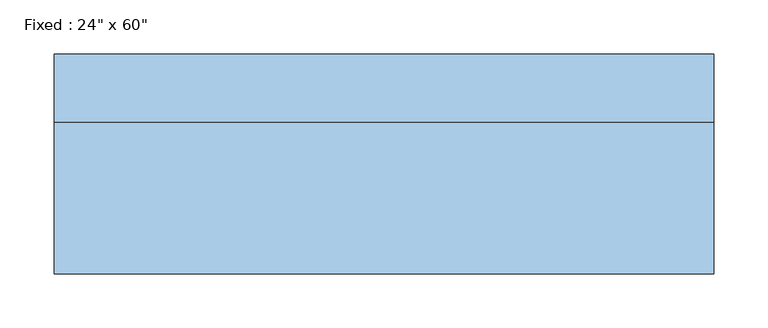
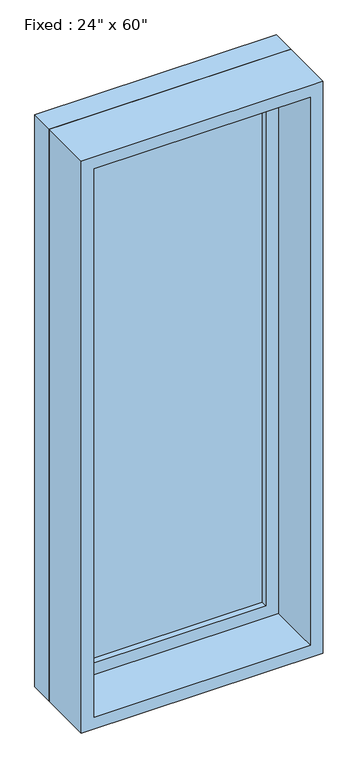
"""IFC4 building model written with IfcOpenShell, lengths in millimetres: window geometry."""

from ifc_helpers import new_model, si_unit, frame, origin, place, context, project, spatial, polyline, outline, extrude, source, transform, mapped, element, save


def window_8561b6b6(model_context):
    return source(origin(), model_context, "Body", "SweptSolid", [
        extrude(outline(polyline([(203.2, 53.975), (-279.4, 53.975), (-279.4, 66.675), (203.2, 66.675), (203.2, 53.975)])), frame((0.0, 0.0, 977.9), z_axis=(0.0, 0.0, 1.0), x_axis=(1.0, 0.0, 0.0)), (0.0, 0.0, 1.0), 1397.0),
        extrude(outline(polyline([(2419.35, -323.85), (933.45, -323.85), (933.45, 247.65), (2419.35, 247.65), (2419.35, -323.85)]), holes=[polyline([(2374.9, -279.4), (2374.9, 203.2), (977.9, 203.2), (977.9, -279.4), (2374.9, -279.4)])]), frame((0.0, 38.1, 0.0), z_axis=(0.0, 1.0, 0.0), x_axis=(0.0, 0.0, 1.0)), (0.0, 0.0, 1.0), 44.45),
        extrude(outline(polyline([(2438.4, -342.9), (914.4, -342.9), (914.4, 266.7), (2438.4, 266.7), (2438.4, -342.9)]), holes=[polyline([(2406.65, -311.15), (2406.65, 234.95), (946.15, 234.95), (946.15, -311.15), (2406.65, -311.15)])]), frame((0.0, -101.6, 0.0), z_axis=(0.0, 1.0, 0.0), x_axis=(0.0, 0.0, 1.0)), (0.0, 0.0, 1.0), 139.7),
        extrude(outline(polyline([(2438.4, 266.7), (2438.4, -342.9), (914.4, -342.9), (914.4, 266.7), (2438.4, 266.7)]), holes=[polyline([(2419.35, 247.65), (933.45, 247.65), (933.45, -323.85), (2419.35, -323.85), (2419.35, 247.65)])]), frame((0.0, 38.1, 0.0), z_axis=(0.0, 1.0, 0.0), x_axis=(0.0, 0.0, 1.0)), (0.0, 0.0, 1.0), 63.5),
    ])


if __name__ == "__main__":
    model = new_model("IFC4")
    model_context = context("Model", 3, world=origin())
    ifc_project = project(units=[si_unit("LENGTHUNIT", "METRE", prefix="MILLI")], contexts=[model_context])
    site = spatial("IfcSite", under=ifc_project)
    building = spatial("IfcBuilding", under=site)
    placement = place(None, origin())
    window_shape = window_8561b6b6(model_context)
    element("IfcWindow", 1, ObjectType="Fixed : 24\" x 60\"", at=placement, inside=building, context=model_context, shape_type="MappedRepresentation", body=[
        mapped(window_shape, transform((0.0, 0.0, 0.0), x_axis=(1.0, 0.0, 0.0), y_axis=(0.0, 1.0, 0.0), z_axis=(0.0, 0.0, 1.0))),
    ])
    save(model, "model.ifc")

# Revit data of these elements
# Type "Fixed : 24\" x 60\""
#   Type Mark = "5"
#   Construction Type Id = "GSP4R"
#   Assembly Code = "B2020100"
#   Analytic Construction = "1/8 in Pilkington single glazing"
#   Visual Light Transmittance = 0.9
#   Solar Heat Gain Coefficient = 0.78
#   Heat Transfer Coefficient (U) = 0.6496 BTU/(h·ft²·°F)
#   Height = 5' - 0"
#   Default Sill Height = 3' - 0"
#   Width = 2' - 0"
#   Window Inset = 0' - 0 3/4"
#   Define Thermal Properties by = 1
#   Glass Pane Material = Glass
#   Sash Material = Sash
#   Wall Closure = (empty or 0)
# Element 1 (IfcWindow, "Fixed : 24\" x 60\"")
#   Materials on its faces: "Sash", "Glass"
# Materials
#   "Glass": class "Glass", colour RGB 0 128 192, transparency 0.75, Description = "Soda Lime Glass", Cost = 0
#   "Sash": class "Wood", colour RGB 224 178 126, transparency 0
